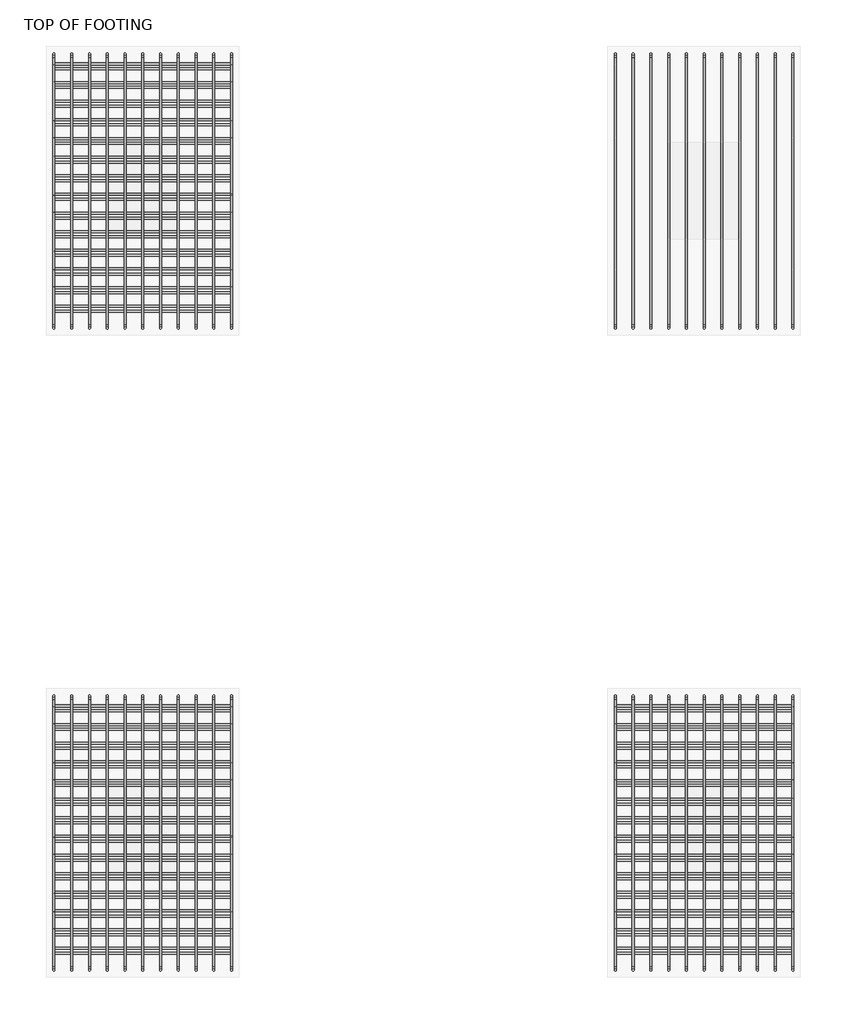
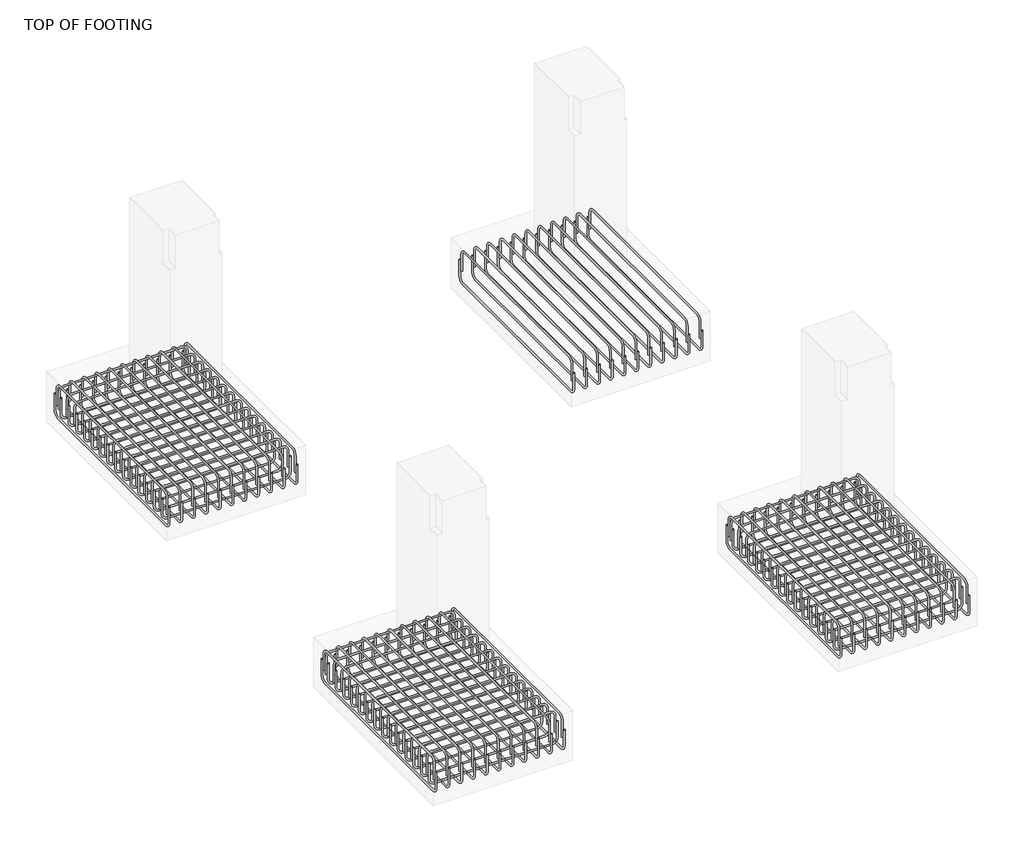
# One storey, part 9 of 11: 14 reinforcing bars.
"""IFC4 building model written with IfcOpenShell, lengths in millimetres."""

from ifc_helpers import new_model, si_unit, point, frame, origin, place, context, project, spatial, polyline, circle_curve, trimmed, segment, composite_curve, source, transform, mapped, element, save
from ifc_brep_helpers import swept_disk

model = new_model("IFC4")

# Units and contexts
model_context = context("Model", 3, world=origin())
ifc_project = project(units=[si_unit("LENGTHUNIT", "METRE", prefix="MILLI")], contexts=[model_context])

# Site, building, storey
site = spatial("IfcSite", under=ifc_project)
building = spatial("IfcBuilding", under=site)
storey = spatial("IfcBuildingStorey", under=building, Name="TOP OF FOOTING", Elevation=-1828.8)

# Reinforcing bars
placement = place(None, origin())
reinforcing_bar_shape = source(origin(), model_context, "Body", "SolidModel", [
    swept_disk(composite_curve([segment(polyline([(5183.7615906, 14549.4712443, -2012.1658531), (5183.7615906, 14549.4712443, -2159.4658531)]), True, "CONTINUOUS"), segment(trimmed(circle_curve(frame((5183.7615906, 14595.8212443, -2159.4658531), z_axis=(1.0, 0.0, 0.0), x_axis=(0.0, -46.349999999998545, 0.0)), 46.35), [point((5183.7615906, 14549.4712443, -2159.4658531))], [point((5183.7615906, 14595.8212443, -2205.8158531))], True, "CARTESIAN"), True, "CONTINUOUS"), segment(polyline([(5183.7615906, 14595.8212443, -2205.8158531), (5183.7615906, 16210.4212443, -2205.8158531)]), True, "CONTINUOUS"), segment(trimmed(circle_curve(frame((5183.7615906, 16210.4212443, -2159.4658531), z_axis=(1.0, 0.0, 0.0), x_axis=(0.0, 0.0, -46.34999999999991)), 46.35), [point((5183.7615906, 16210.4212443, -2205.8158531))], [point((5183.7615906, 16256.7712443, -2159.4658531))], True, "CARTESIAN"), True, "CONTINUOUS"), segment(polyline([(5183.7615906, 16256.7712443, -2159.4658531), (5183.7615906, 16256.7712443, -2012.1658531)]), True, "CONTINUOUS")], self_intersect=False), 6.35),
])
element("IfcReinforcingBar", 1, at=placement, inside=storey, context=model_context, shape_type="MappedRepresentation", body=[
    mapped(reinforcing_bar_shape, transform((0.0, 0.0, 0.0), x_axis=(1.0, 0.0, 0.0), y_axis=(0.0, 1.0, 0.0), z_axis=(0.0, 0.0, 1.0))),
    mapped(reinforcing_bar_shape, transform((-110.73, 0.0, 0.0), x_axis=(1.0, 0.0, 0.0), y_axis=(0.0, 1.0, 0.0), z_axis=(0.0, 0.0, 1.0))),
    mapped(reinforcing_bar_shape, transform((-221.46, 0.0, 0.0), x_axis=(1.0, 0.0, 0.0), y_axis=(0.0, 1.0, 0.0), z_axis=(0.0, 0.0, 1.0))),
    mapped(reinforcing_bar_shape, transform((-332.19, 0.0, 0.0), x_axis=(1.0, 0.0, 0.0), y_axis=(0.0, 1.0, 0.0), z_axis=(0.0, 0.0, 1.0))),
    mapped(reinforcing_bar_shape, transform((-442.92, 0.0, 0.0), x_axis=(1.0, 0.0, 0.0), y_axis=(0.0, 1.0, 0.0), z_axis=(0.0, 0.0, 1.0))),
    mapped(reinforcing_bar_shape, transform((-553.65, 0.0, 0.0), x_axis=(1.0, 0.0, 0.0), y_axis=(0.0, 1.0, 0.0), z_axis=(0.0, 0.0, 1.0))),
    mapped(reinforcing_bar_shape, transform((-664.38, 0.0, 0.0), x_axis=(1.0, 0.0, 0.0), y_axis=(0.0, 1.0, 0.0), z_axis=(0.0, 0.0, 1.0))),
    mapped(reinforcing_bar_shape, transform((-775.11, 0.0, 0.0), x_axis=(1.0, 0.0, 0.0), y_axis=(0.0, 1.0, 0.0), z_axis=(0.0, 0.0, 1.0))),
    mapped(reinforcing_bar_shape, transform((-885.84, 0.0, 0.0), x_axis=(1.0, 0.0, 0.0), y_axis=(0.0, 1.0, 0.0), z_axis=(0.0, 0.0, 1.0))),
    mapped(reinforcing_bar_shape, transform((-996.57, 0.0, 0.0), x_axis=(1.0, 0.0, 0.0), y_axis=(0.0, 1.0, 0.0), z_axis=(0.0, 0.0, 1.0))),
    mapped(reinforcing_bar_shape, transform((-1107.3, 0.0, 0.0), x_axis=(1.0, 0.0, 0.0), y_axis=(0.0, 1.0, 0.0), z_axis=(0.0, 0.0, 1.0))),
])
reinforcing_bar_2_shape = source(origin(), model_context, "Body", "SolidModel", [
    swept_disk(composite_curve([segment(polyline([(4076.4615906, 14577.6603603, -2096.8914539), (4076.4615906, 14577.6603603, -1949.5914539)]), True, "CONTINUOUS"), segment(trimmed(circle_curve(frame((4076.4615906, 14624.0103603, -1949.5914539), z_axis=(-1.0, 0.0, 0.0), x_axis=(0.0, -46.350000000000364, 0.0)), 46.35), [point((4076.4615906, 14577.6603603, -1949.5914539))], [point((4076.4615906, 14624.0103603, -1903.2414539))], True, "CARTESIAN"), True, "CONTINUOUS"), segment(polyline([(4076.4615906, 14624.0103603, -1903.2414539), (4076.4615906, 16181.3238837, -1903.2414539)]), True, "CONTINUOUS"), segment(trimmed(circle_curve(frame((4076.4615906, 16181.3238837, -1949.5914539), z_axis=(-1.0, 0.0, 0.0), x_axis=(0.0, 0.0, 46.350000000000136)), 46.35), [point((4076.4615906, 16181.3238837, -1903.2414539))], [point((4076.4615906, 16227.6738837, -1949.5914539))], True, "CARTESIAN"), True, "CONTINUOUS"), segment(polyline([(4076.4615906, 16227.6738837, -1949.5914539), (4076.4615906, 16227.6738837, -2096.8914539)]), True, "CONTINUOUS")], self_intersect=False), 6.35),
])
element("IfcReinforcingBar", 2, at=placement, inside=storey, context=model_context, shape_type="MappedRepresentation", body=[
    mapped(reinforcing_bar_2_shape, transform((0.0, 0.0, 0.0), x_axis=(1.0, 0.0, 0.0), y_axis=(0.0, 1.0, 0.0), z_axis=(0.0, 0.0, 1.0))),
    mapped(reinforcing_bar_2_shape, transform((110.73, 0.0, 0.0), x_axis=(1.0, 0.0, 0.0), y_axis=(0.0, 1.0, 0.0), z_axis=(0.0, 0.0, 1.0))),
    mapped(reinforcing_bar_2_shape, transform((221.46, 0.0, 0.0), x_axis=(1.0, 0.0, 0.0), y_axis=(0.0, 1.0, 0.0), z_axis=(0.0, 0.0, 1.0))),
    mapped(reinforcing_bar_2_shape, transform((332.19, 0.0, 0.0), x_axis=(1.0, 0.0, 0.0), y_axis=(0.0, 1.0, 0.0), z_axis=(0.0, 0.0, 1.0))),
    mapped(reinforcing_bar_2_shape, transform((442.92, 0.0, 0.0), x_axis=(1.0, 0.0, 0.0), y_axis=(0.0, 1.0, 0.0), z_axis=(0.0, 0.0, 1.0))),
    mapped(reinforcing_bar_2_shape, transform((553.65, 0.0, 0.0), x_axis=(1.0, 0.0, 0.0), y_axis=(0.0, 1.0, 0.0), z_axis=(0.0, 0.0, 1.0))),
    mapped(reinforcing_bar_2_shape, transform((664.38, 0.0, 0.0), x_axis=(1.0, 0.0, 0.0), y_axis=(0.0, 1.0, 0.0), z_axis=(0.0, 0.0, 1.0))),
    mapped(reinforcing_bar_2_shape, transform((775.11, 0.0, 0.0), x_axis=(1.0, 0.0, 0.0), y_axis=(0.0, 1.0, 0.0), z_axis=(0.0, 0.0, 1.0))),
    mapped(reinforcing_bar_2_shape, transform((885.84, 0.0, 0.0), x_axis=(1.0, 0.0, 0.0), y_axis=(0.0, 1.0, 0.0), z_axis=(0.0, 0.0, 1.0))),
    mapped(reinforcing_bar_2_shape, transform((996.57, 0.0, 0.0), x_axis=(1.0, 0.0, 0.0), y_axis=(0.0, 1.0, 0.0), z_axis=(0.0, 0.0, 1.0))),
    mapped(reinforcing_bar_2_shape, transform((1107.3, 0.0, 0.0), x_axis=(1.0, 0.0, 0.0), y_axis=(0.0, 1.0, 0.0), z_axis=(0.0, 0.0, 1.0))),
])
reinforcing_bar_3_shape = source(origin(), model_context, "Body", "SolidModel", [
    swept_disk(composite_curve([segment(polyline([(5183.7615906, 10549.4712443, -2012.1658531), (5183.7615906, 10549.4712443, -2159.4658531)]), True, "CONTINUOUS"), segment(trimmed(circle_curve(frame((5183.7615906, 10595.8212443, -2159.4658531), z_axis=(1.0, 0.0, 0.0), x_axis=(0.0, -46.349999999998545, 0.0)), 46.35), [point((5183.7615906, 10549.4712443, -2159.4658531))], [point((5183.7615906, 10595.8212443, -2205.8158531))], True, "CARTESIAN"), True, "CONTINUOUS"), segment(polyline([(5183.7615906, 10595.8212443, -2205.8158531), (5183.7615906, 12210.4212443, -2205.8158531)]), True, "CONTINUOUS"), segment(trimmed(circle_curve(frame((5183.7615906, 12210.4212443, -2159.4658531), z_axis=(1.0, 0.0, 0.0), x_axis=(0.0, 0.0, -46.34999999999991)), 46.35), [point((5183.7615906, 12210.4212443, -2205.8158531))], [point((5183.7615906, 12256.7712443, -2159.4658531))], True, "CARTESIAN"), True, "CONTINUOUS"), segment(polyline([(5183.7615906, 12256.7712443, -2159.4658531), (5183.7615906, 12256.7712443, -2012.1658531)]), True, "CONTINUOUS")], self_intersect=False), 6.35),
])
element("IfcReinforcingBar", 3, at=placement, inside=storey, context=model_context, shape_type="MappedRepresentation", body=[
    mapped(reinforcing_bar_3_shape, transform((0.0, 0.0, 0.0), x_axis=(1.0, 0.0, 0.0), y_axis=(0.0, 1.0, 0.0), z_axis=(0.0, 0.0, 1.0))),
    mapped(reinforcing_bar_3_shape, transform((-110.73, 0.0, 0.0), x_axis=(1.0, 0.0, 0.0), y_axis=(0.0, 1.0, 0.0), z_axis=(0.0, 0.0, 1.0))),
    mapped(reinforcing_bar_3_shape, transform((-221.46, 0.0, 0.0), x_axis=(1.0, 0.0, 0.0), y_axis=(0.0, 1.0, 0.0), z_axis=(0.0, 0.0, 1.0))),
    mapped(reinforcing_bar_3_shape, transform((-332.19, 0.0, 0.0), x_axis=(1.0, 0.0, 0.0), y_axis=(0.0, 1.0, 0.0), z_axis=(0.0, 0.0, 1.0))),
    mapped(reinforcing_bar_3_shape, transform((-442.92, 0.0, 0.0), x_axis=(1.0, 0.0, 0.0), y_axis=(0.0, 1.0, 0.0), z_axis=(0.0, 0.0, 1.0))),
    mapped(reinforcing_bar_3_shape, transform((-553.65, 0.0, 0.0), x_axis=(1.0, 0.0, 0.0), y_axis=(0.0, 1.0, 0.0), z_axis=(0.0, 0.0, 1.0))),
    mapped(reinforcing_bar_3_shape, transform((-664.38, 0.0, 0.0), x_axis=(1.0, 0.0, 0.0), y_axis=(0.0, 1.0, 0.0), z_axis=(0.0, 0.0, 1.0))),
    mapped(reinforcing_bar_3_shape, transform((-775.11, 0.0, 0.0), x_axis=(1.0, 0.0, 0.0), y_axis=(0.0, 1.0, 0.0), z_axis=(0.0, 0.0, 1.0))),
    mapped(reinforcing_bar_3_shape, transform((-885.84, 0.0, 0.0), x_axis=(1.0, 0.0, 0.0), y_axis=(0.0, 1.0, 0.0), z_axis=(0.0, 0.0, 1.0))),
    mapped(reinforcing_bar_3_shape, transform((-996.57, 0.0, 0.0), x_axis=(1.0, 0.0, 0.0), y_axis=(0.0, 1.0, 0.0), z_axis=(0.0, 0.0, 1.0))),
    mapped(reinforcing_bar_3_shape, transform((-1107.3, 0.0, 0.0), x_axis=(1.0, 0.0, 0.0), y_axis=(0.0, 1.0, 0.0), z_axis=(0.0, 0.0, 1.0))),
])
reinforcing_bar_4_shape = source(origin(), model_context, "Body", "SolidModel", [
    swept_disk(composite_curve([segment(polyline([(4076.4615906, 10577.6603603, -2096.8914539), (4076.4615906, 10577.6603603, -1949.5914539)]), True, "CONTINUOUS"), segment(trimmed(circle_curve(frame((4076.4615906, 10624.0103603, -1949.5914539), z_axis=(-1.0, 0.0, 0.0), x_axis=(0.0, -46.350000000000364, 0.0)), 46.35), [point((4076.4615906, 10577.6603603, -1949.5914539))], [point((4076.4615906, 10624.0103603, -1903.2414539))], True, "CARTESIAN"), True, "CONTINUOUS"), segment(polyline([(4076.4615906, 10624.0103603, -1903.2414539), (4076.4615906, 12181.3238837, -1903.2414539)]), True, "CONTINUOUS"), segment(trimmed(circle_curve(frame((4076.4615906, 12181.3238837, -1949.5914539), z_axis=(-1.0, 0.0, 0.0), x_axis=(0.0, 0.0, 46.350000000000136)), 46.35), [point((4076.4615906, 12181.3238837, -1903.2414539))], [point((4076.4615906, 12227.6738837, -1949.5914539))], True, "CARTESIAN"), True, "CONTINUOUS"), segment(polyline([(4076.4615906, 12227.6738837, -1949.5914539), (4076.4615906, 12227.6738837, -2096.8914539)]), True, "CONTINUOUS")], self_intersect=False), 6.35),
])
element("IfcReinforcingBar", 4, at=placement, inside=storey, context=model_context, shape_type="MappedRepresentation", body=[
    mapped(reinforcing_bar_4_shape, transform((0.0, 0.0, 0.0), x_axis=(1.0, 0.0, 0.0), y_axis=(0.0, 1.0, 0.0), z_axis=(0.0, 0.0, 1.0))),
    mapped(reinforcing_bar_4_shape, transform((110.73, 0.0, 0.0), x_axis=(1.0, 0.0, 0.0), y_axis=(0.0, 1.0, 0.0), z_axis=(0.0, 0.0, 1.0))),
    mapped(reinforcing_bar_4_shape, transform((221.46, 0.0, 0.0), x_axis=(1.0, 0.0, 0.0), y_axis=(0.0, 1.0, 0.0), z_axis=(0.0, 0.0, 1.0))),
    mapped(reinforcing_bar_4_shape, transform((332.19, 0.0, 0.0), x_axis=(1.0, 0.0, 0.0), y_axis=(0.0, 1.0, 0.0), z_axis=(0.0, 0.0, 1.0))),
    mapped(reinforcing_bar_4_shape, transform((442.92, 0.0, 0.0), x_axis=(1.0, 0.0, 0.0), y_axis=(0.0, 1.0, 0.0), z_axis=(0.0, 0.0, 1.0))),
    mapped(reinforcing_bar_4_shape, transform((553.65, 0.0, 0.0), x_axis=(1.0, 0.0, 0.0), y_axis=(0.0, 1.0, 0.0), z_axis=(0.0, 0.0, 1.0))),
    mapped(reinforcing_bar_4_shape, transform((664.38, 0.0, 0.0), x_axis=(1.0, 0.0, 0.0), y_axis=(0.0, 1.0, 0.0), z_axis=(0.0, 0.0, 1.0))),
    mapped(reinforcing_bar_4_shape, transform((775.11, 0.0, 0.0), x_axis=(1.0, 0.0, 0.0), y_axis=(0.0, 1.0, 0.0), z_axis=(0.0, 0.0, 1.0))),
    mapped(reinforcing_bar_4_shape, transform((885.84, 0.0, 0.0), x_axis=(1.0, 0.0, 0.0), y_axis=(0.0, 1.0, 0.0), z_axis=(0.0, 0.0, 1.0))),
    mapped(reinforcing_bar_4_shape, transform((996.57, 0.0, 0.0), x_axis=(1.0, 0.0, 0.0), y_axis=(0.0, 1.0, 0.0), z_axis=(0.0, 0.0, 1.0))),
    mapped(reinforcing_bar_4_shape, transform((1107.3, 0.0, 0.0), x_axis=(1.0, 0.0, 0.0), y_axis=(0.0, 1.0, 0.0), z_axis=(0.0, 0.0, 1.0))),
])
reinforcing_bar_5_shape = source(origin(), model_context, "Body", "SolidModel", [
    swept_disk(composite_curve([segment(polyline([(4076.4615906, 10653.1930221, -1996.7664426), (4076.4615906, 10653.1930221, -2144.0664426)]), True, "CONTINUOUS"), segment(trimmed(circle_curve(frame((4122.8115906, 10653.1930221, -2144.0664426), z_axis=(0.0, -1.0, 0.0), x_axis=(-46.350000000000364, 0.0, 0.0)), 46.35), [point((4076.4615906, 10653.1930221, -2144.0664426))], [point((4122.8115906, 10653.1930221, -2190.4164426))], True, "CARTESIAN"), True, "CONTINUOUS"), segment(polyline([(4122.8115906, 10653.1930221, -2190.4164426), (5137.4115906, 10653.1930221, -2190.4164426)]), True, "CONTINUOUS"), segment(trimmed(circle_curve(frame((5137.4115906, 10653.1930221, -2144.0664426), z_axis=(0.0, -1.0, 0.0), x_axis=(0.0, 0.0, -46.350000000000364)), 46.35), [point((5137.4115906, 10653.1930221, -2190.4164426))], [point((5183.7615906, 10653.1930221, -2144.0664426))], True, "CARTESIAN"), True, "CONTINUOUS"), segment(polyline([(5183.7615906, 10653.1930221, -2144.0664426), (5183.7615906, 10653.1930221, -1996.7664426)]), True, "CONTINUOUS")], self_intersect=False), 6.35),
])
element("IfcReinforcingBar", 5, at=placement, inside=storey, context=model_context, shape_type="MappedRepresentation", body=[
    mapped(reinforcing_bar_5_shape, transform((0.0, 0.0, 0.0), x_axis=(1.0, 0.0, 0.0), y_axis=(0.0, 1.0, 0.0), z_axis=(0.0, 0.0, 1.0))),
    mapped(reinforcing_bar_5_shape, transform((0.0, 116.2744005, 0.0), x_axis=(1.0, 0.0, 0.0), y_axis=(0.0, 1.0, 0.0), z_axis=(0.0, 0.0, 1.0))),
    mapped(reinforcing_bar_5_shape, transform((0.0, 232.5488009, 0.0), x_axis=(1.0, 0.0, 0.0), y_axis=(0.0, 1.0, 0.0), z_axis=(0.0, 0.0, 1.0))),
    mapped(reinforcing_bar_5_shape, transform((0.0, 348.8232014, 0.0), x_axis=(1.0, 0.0, 0.0), y_axis=(0.0, 1.0, 0.0), z_axis=(0.0, 0.0, 1.0))),
    mapped(reinforcing_bar_5_shape, transform((0.0, 465.0976018, 0.0), x_axis=(1.0, 0.0, 0.0), y_axis=(0.0, 1.0, 0.0), z_axis=(0.0, 0.0, 1.0))),
    mapped(reinforcing_bar_5_shape, transform((0.0, 581.3720023, 0.0), x_axis=(1.0, 0.0, 0.0), y_axis=(0.0, 1.0, 0.0), z_axis=(0.0, 0.0, 1.0))),
    mapped(reinforcing_bar_5_shape, transform((0.0, 697.6464027, 0.0), x_axis=(1.0, 0.0, 0.0), y_axis=(0.0, 1.0, 0.0), z_axis=(0.0, 0.0, 1.0))),
    mapped(reinforcing_bar_5_shape, transform((0.0, 813.9208032, 0.0), x_axis=(1.0, 0.0, 0.0), y_axis=(0.0, 1.0, 0.0), z_axis=(0.0, 0.0, 1.0))),
    mapped(reinforcing_bar_5_shape, transform((0.0, 930.1952036, 0.0), x_axis=(1.0, 0.0, 0.0), y_axis=(0.0, 1.0, 0.0), z_axis=(0.0, 0.0, 1.0))),
    mapped(reinforcing_bar_5_shape, transform((0.0, 1046.4696041, 0.0), x_axis=(1.0, 0.0, 0.0), y_axis=(0.0, 1.0, 0.0), z_axis=(0.0, 0.0, 1.0))),
    mapped(reinforcing_bar_5_shape, transform((0.0, 1162.7440045, 0.0), x_axis=(1.0, 0.0, 0.0), y_axis=(0.0, 1.0, 0.0), z_axis=(0.0, 0.0, 1.0))),
    mapped(reinforcing_bar_5_shape, transform((0.0, 1279.018405, 0.0), x_axis=(1.0, 0.0, 0.0), y_axis=(0.0, 1.0, 0.0), z_axis=(0.0, 0.0, 1.0))),
    mapped(reinforcing_bar_5_shape, transform((0.0, 1395.2928054, 0.0), x_axis=(1.0, 0.0, 0.0), y_axis=(0.0, 1.0, 0.0), z_axis=(0.0, 0.0, 1.0))),
    mapped(reinforcing_bar_5_shape, transform((0.0, 1511.5672059, 0.0), x_axis=(1.0, 0.0, 0.0), y_axis=(0.0, 1.0, 0.0), z_axis=(0.0, 0.0, 1.0))),
])
reinforcing_bar_6_shape = source(origin(), model_context, "Body", "SolidModel", [
    swept_disk(composite_curve([segment(polyline([(4076.4615906, 12194.4257435, -2114.1958609), (4076.4615906, 12194.4257435, -1966.8958609)]), True, "CONTINUOUS"), segment(trimmed(circle_curve(frame((4122.8115906, 12194.4257435, -1966.8958609), z_axis=(0.0, 1.0, 0.0), x_axis=(-46.350000000000364, 0.0, 0.0)), 46.35), [point((4076.4615906, 12194.4257435, -1966.8958609))], [point((4122.8115906, 12194.4257435, -1920.5458609))], True, "CARTESIAN"), True, "CONTINUOUS"), segment(polyline([(4122.8115906, 12194.4257435, -1920.5458609), (5137.4115906, 12194.4257435, -1920.5458609)]), True, "CONTINUOUS"), segment(trimmed(circle_curve(frame((5137.4115906, 12194.4257435, -1966.8958609), z_axis=(0.0, 1.0, 0.0), x_axis=(0.0, 0.0, 46.34999999999991)), 46.35), [point((5137.4115906, 12194.4257435, -1920.5458609))], [point((5183.7615906, 12194.4257435, -1966.8958609))], True, "CARTESIAN"), True, "CONTINUOUS"), segment(polyline([(5183.7615906, 12194.4257435, -1966.8958609), (5183.7615906, 12194.4257435, -2114.1958609)]), True, "CONTINUOUS")], self_intersect=False), 6.35),
])
element("IfcReinforcingBar", 6, at=placement, inside=storey, context=model_context, shape_type="MappedRepresentation", body=[
    mapped(reinforcing_bar_6_shape, transform((0.0, 0.0, 0.0), x_axis=(1.0, 0.0, 0.0), y_axis=(0.0, 1.0, 0.0), z_axis=(0.0, 0.0, 1.0))),
    mapped(reinforcing_bar_6_shape, transform((0.0, -116.1057918, 0.0), x_axis=(1.0, 0.0, 0.0), y_axis=(0.0, 1.0, 0.0), z_axis=(0.0, 0.0, 1.0))),
    mapped(reinforcing_bar_6_shape, transform((0.0, -232.2115836, 0.0), x_axis=(1.0, 0.0, 0.0), y_axis=(0.0, 1.0, 0.0), z_axis=(0.0, 0.0, 1.0))),
    mapped(reinforcing_bar_6_shape, transform((0.0, -348.3173754, 0.0), x_axis=(1.0, 0.0, 0.0), y_axis=(0.0, 1.0, 0.0), z_axis=(0.0, 0.0, 1.0))),
    mapped(reinforcing_bar_6_shape, transform((0.0, -464.4231672, 0.0), x_axis=(1.0, 0.0, 0.0), y_axis=(0.0, 1.0, 0.0), z_axis=(0.0, 0.0, 1.0))),
    mapped(reinforcing_bar_6_shape, transform((0.0, -580.528959, 0.0), x_axis=(1.0, 0.0, 0.0), y_axis=(0.0, 1.0, 0.0), z_axis=(0.0, 0.0, 1.0))),
    mapped(reinforcing_bar_6_shape, transform((0.0, -696.6347508, 0.0), x_axis=(1.0, 0.0, 0.0), y_axis=(0.0, 1.0, 0.0), z_axis=(0.0, 0.0, 1.0))),
    mapped(reinforcing_bar_6_shape, transform((0.0, -812.7405426, 0.0), x_axis=(1.0, 0.0, 0.0), y_axis=(0.0, 1.0, 0.0), z_axis=(0.0, 0.0, 1.0))),
    mapped(reinforcing_bar_6_shape, transform((0.0, -928.8463344, 0.0), x_axis=(1.0, 0.0, 0.0), y_axis=(0.0, 1.0, 0.0), z_axis=(0.0, 0.0, 1.0))),
    mapped(reinforcing_bar_6_shape, transform((0.0, -1044.9521262, 0.0), x_axis=(1.0, 0.0, 0.0), y_axis=(0.0, 1.0, 0.0), z_axis=(0.0, 0.0, 1.0))),
    mapped(reinforcing_bar_6_shape, transform((0.0, -1161.057918, 0.0), x_axis=(1.0, 0.0, 0.0), y_axis=(0.0, 1.0, 0.0), z_axis=(0.0, 0.0, 1.0))),
    mapped(reinforcing_bar_6_shape, transform((0.0, -1277.1637098, 0.0), x_axis=(1.0, 0.0, 0.0), y_axis=(0.0, 1.0, 0.0), z_axis=(0.0, 0.0, 1.0))),
    mapped(reinforcing_bar_6_shape, transform((0.0, -1393.2695016, 0.0), x_axis=(1.0, 0.0, 0.0), y_axis=(0.0, 1.0, 0.0), z_axis=(0.0, 0.0, 1.0))),
    mapped(reinforcing_bar_6_shape, transform((0.0, -1509.3752934, 0.0), x_axis=(1.0, 0.0, 0.0), y_axis=(0.0, 1.0, 0.0), z_axis=(0.0, 0.0, 1.0))),
])
reinforcing_bar_7_shape = source(origin(), model_context, "Body", "SolidModel", [
    swept_disk(composite_curve([segment(polyline([(1683.7615906, 14549.4712443, -2012.1658531), (1683.7615906, 14549.4712443, -2159.4658531)]), True, "CONTINUOUS"), segment(trimmed(circle_curve(frame((1683.7615906, 14595.8212443, -2159.4658531), z_axis=(1.0, 0.0, 0.0), x_axis=(0.0, -46.349999999998545, 0.0)), 46.35), [point((1683.7615906, 14549.4712443, -2159.4658531))], [point((1683.7615906, 14595.8212443, -2205.8158531))], True, "CARTESIAN"), True, "CONTINUOUS"), segment(polyline([(1683.7615906, 14595.8212443, -2205.8158531), (1683.7615906, 16210.4212443, -2205.8158531)]), True, "CONTINUOUS"), segment(trimmed(circle_curve(frame((1683.7615906, 16210.4212443, -2159.4658531), z_axis=(1.0, 0.0, 0.0), x_axis=(0.0, 0.0, -46.34999999999991)), 46.35), [point((1683.7615906, 16210.4212443, -2205.8158531))], [point((1683.7615906, 16256.7712443, -2159.4658531))], True, "CARTESIAN"), True, "CONTINUOUS"), segment(polyline([(1683.7615906, 16256.7712443, -2159.4658531), (1683.7615906, 16256.7712443, -2012.1658531)]), True, "CONTINUOUS")], self_intersect=False), 6.35),
])
element("IfcReinforcingBar", 7, at=placement, inside=storey, context=model_context, shape_type="MappedRepresentation", body=[
    mapped(reinforcing_bar_7_shape, transform((0.0, 0.0, 0.0), x_axis=(1.0, 0.0, 0.0), y_axis=(0.0, 1.0, 0.0), z_axis=(0.0, 0.0, 1.0))),
    mapped(reinforcing_bar_7_shape, transform((-110.73, 0.0, 0.0), x_axis=(1.0, 0.0, 0.0), y_axis=(0.0, 1.0, 0.0), z_axis=(0.0, 0.0, 1.0))),
    mapped(reinforcing_bar_7_shape, transform((-221.46, 0.0, 0.0), x_axis=(1.0, 0.0, 0.0), y_axis=(0.0, 1.0, 0.0), z_axis=(0.0, 0.0, 1.0))),
    mapped(reinforcing_bar_7_shape, transform((-332.19, 0.0, 0.0), x_axis=(1.0, 0.0, 0.0), y_axis=(0.0, 1.0, 0.0), z_axis=(0.0, 0.0, 1.0))),
    mapped(reinforcing_bar_7_shape, transform((-442.92, 0.0, 0.0), x_axis=(1.0, 0.0, 0.0), y_axis=(0.0, 1.0, 0.0), z_axis=(0.0, 0.0, 1.0))),
    mapped(reinforcing_bar_7_shape, transform((-553.65, 0.0, 0.0), x_axis=(1.0, 0.0, 0.0), y_axis=(0.0, 1.0, 0.0), z_axis=(0.0, 0.0, 1.0))),
    mapped(reinforcing_bar_7_shape, transform((-664.38, 0.0, 0.0), x_axis=(1.0, 0.0, 0.0), y_axis=(0.0, 1.0, 0.0), z_axis=(0.0, 0.0, 1.0))),
    mapped(reinforcing_bar_7_shape, transform((-775.11, 0.0, 0.0), x_axis=(1.0, 0.0, 0.0), y_axis=(0.0, 1.0, 0.0), z_axis=(0.0, 0.0, 1.0))),
    mapped(reinforcing_bar_7_shape, transform((-885.84, 0.0, 0.0), x_axis=(1.0, 0.0, 0.0), y_axis=(0.0, 1.0, 0.0), z_axis=(0.0, 0.0, 1.0))),
    mapped(reinforcing_bar_7_shape, transform((-996.57, 0.0, 0.0), x_axis=(1.0, 0.0, 0.0), y_axis=(0.0, 1.0, 0.0), z_axis=(0.0, 0.0, 1.0))),
    mapped(reinforcing_bar_7_shape, transform((-1107.3, 0.0, 0.0), x_axis=(1.0, 0.0, 0.0), y_axis=(0.0, 1.0, 0.0), z_axis=(0.0, 0.0, 1.0))),
])
reinforcing_bar_8_shape = source(origin(), model_context, "Body", "SolidModel", [
    swept_disk(composite_curve([segment(polyline([(576.4615906, 14577.6603603, -2096.8914539), (576.4615906, 14577.6603603, -1949.5914539)]), True, "CONTINUOUS"), segment(trimmed(circle_curve(frame((576.4615906, 14624.0103603, -1949.5914539), z_axis=(-1.0, 0.0, 0.0), x_axis=(0.0, -46.350000000000364, 0.0)), 46.35), [point((576.4615906, 14577.6603603, -1949.5914539))], [point((576.4615906, 14624.0103603, -1903.2414539))], True, "CARTESIAN"), True, "CONTINUOUS"), segment(polyline([(576.4615906, 14624.0103603, -1903.2414539), (576.4615906, 16181.3238837, -1903.2414539)]), True, "CONTINUOUS"), segment(trimmed(circle_curve(frame((576.4615906, 16181.3238837, -1949.5914539), z_axis=(-1.0, 0.0, 0.0), x_axis=(0.0, 0.0, 46.350000000000136)), 46.35), [point((576.4615906, 16181.3238837, -1903.2414539))], [point((576.4615906, 16227.6738837, -1949.5914539))], True, "CARTESIAN"), True, "CONTINUOUS"), segment(polyline([(576.4615906, 16227.6738837, -1949.5914539), (576.4615906, 16227.6738837, -2096.8914539)]), True, "CONTINUOUS")], self_intersect=False), 6.35),
])
element("IfcReinforcingBar", 8, at=placement, inside=storey, context=model_context, shape_type="MappedRepresentation", body=[
    mapped(reinforcing_bar_8_shape, transform((0.0, 0.0, 0.0), x_axis=(1.0, 0.0, 0.0), y_axis=(0.0, 1.0, 0.0), z_axis=(0.0, 0.0, 1.0))),
    mapped(reinforcing_bar_8_shape, transform((110.73, 0.0, 0.0), x_axis=(1.0, 0.0, 0.0), y_axis=(0.0, 1.0, 0.0), z_axis=(0.0, 0.0, 1.0))),
    mapped(reinforcing_bar_8_shape, transform((221.46, 0.0, 0.0), x_axis=(1.0, 0.0, 0.0), y_axis=(0.0, 1.0, 0.0), z_axis=(0.0, 0.0, 1.0))),
    mapped(reinforcing_bar_8_shape, transform((332.19, 0.0, 0.0), x_axis=(1.0, 0.0, 0.0), y_axis=(0.0, 1.0, 0.0), z_axis=(0.0, 0.0, 1.0))),
    mapped(reinforcing_bar_8_shape, transform((442.92, 0.0, 0.0), x_axis=(1.0, 0.0, 0.0), y_axis=(0.0, 1.0, 0.0), z_axis=(0.0, 0.0, 1.0))),
    mapped(reinforcing_bar_8_shape, transform((553.65, 0.0, 0.0), x_axis=(1.0, 0.0, 0.0), y_axis=(0.0, 1.0, 0.0), z_axis=(0.0, 0.0, 1.0))),
    mapped(reinforcing_bar_8_shape, transform((664.38, 0.0, 0.0), x_axis=(1.0, 0.0, 0.0), y_axis=(0.0, 1.0, 0.0), z_axis=(0.0, 0.0, 1.0))),
    mapped(reinforcing_bar_8_shape, transform((775.11, 0.0, 0.0), x_axis=(1.0, 0.0, 0.0), y_axis=(0.0, 1.0, 0.0), z_axis=(0.0, 0.0, 1.0))),
    mapped(reinforcing_bar_8_shape, transform((885.84, 0.0, 0.0), x_axis=(1.0, 0.0, 0.0), y_axis=(0.0, 1.0, 0.0), z_axis=(0.0, 0.0, 1.0))),
    mapped(reinforcing_bar_8_shape, transform((996.57, 0.0, 0.0), x_axis=(1.0, 0.0, 0.0), y_axis=(0.0, 1.0, 0.0), z_axis=(0.0, 0.0, 1.0))),
    mapped(reinforcing_bar_8_shape, transform((1107.3, 0.0, 0.0), x_axis=(1.0, 0.0, 0.0), y_axis=(0.0, 1.0, 0.0), z_axis=(0.0, 0.0, 1.0))),
])
reinforcing_bar_9_shape = source(origin(), model_context, "Body", "SolidModel", [
    swept_disk(composite_curve([segment(polyline([(576.4615906, 14653.1930221, -1996.7664426), (576.4615906, 14653.1930221, -2144.0664426)]), True, "CONTINUOUS"), segment(trimmed(circle_curve(frame((622.8115906, 14653.1930221, -2144.0664426), z_axis=(0.0, -1.0, 0.0), x_axis=(-46.35000000000002, 0.0, 0.0)), 46.35), [point((576.4615906, 14653.1930221, -2144.0664426))], [point((622.8115906, 14653.1930221, -2190.4164426))], True, "CARTESIAN"), True, "CONTINUOUS"), segment(polyline([(622.8115906, 14653.1930221, -2190.4164426), (1637.4115906, 14653.1930221, -2190.4164426)]), True, "CONTINUOUS"), segment(trimmed(circle_curve(frame((1637.4115906, 14653.1930221, -2144.0664426), z_axis=(0.0, -1.0, 0.0), x_axis=(0.0, 0.0, -46.350000000000364)), 46.35), [point((1637.4115906, 14653.1930221, -2190.4164426))], [point((1683.7615906, 14653.1930221, -2144.0664426))], True, "CARTESIAN"), True, "CONTINUOUS"), segment(polyline([(1683.7615906, 14653.1930221, -2144.0664426), (1683.7615906, 14653.1930221, -1996.7664426)]), True, "CONTINUOUS")], self_intersect=False), 6.35),
])
element("IfcReinforcingBar", 9, at=placement, inside=storey, context=model_context, shape_type="MappedRepresentation", body=[
    mapped(reinforcing_bar_9_shape, transform((0.0, 0.0, 0.0), x_axis=(1.0, 0.0, 0.0), y_axis=(0.0, 1.0, 0.0), z_axis=(0.0, 0.0, 1.0))),
    mapped(reinforcing_bar_9_shape, transform((0.0, 116.2744005, 0.0), x_axis=(1.0, 0.0, 0.0), y_axis=(0.0, 1.0, 0.0), z_axis=(0.0, 0.0, 1.0))),
    mapped(reinforcing_bar_9_shape, transform((0.0, 232.5488009, 0.0), x_axis=(1.0, 0.0, 0.0), y_axis=(0.0, 1.0, 0.0), z_axis=(0.0, 0.0, 1.0))),
    mapped(reinforcing_bar_9_shape, transform((0.0, 348.8232014, 0.0), x_axis=(1.0, 0.0, 0.0), y_axis=(0.0, 1.0, 0.0), z_axis=(0.0, 0.0, 1.0))),
    mapped(reinforcing_bar_9_shape, transform((0.0, 465.0976018, 0.0), x_axis=(1.0, 0.0, 0.0), y_axis=(0.0, 1.0, 0.0), z_axis=(0.0, 0.0, 1.0))),
    mapped(reinforcing_bar_9_shape, transform((0.0, 581.3720023, 0.0), x_axis=(1.0, 0.0, 0.0), y_axis=(0.0, 1.0, 0.0), z_axis=(0.0, 0.0, 1.0))),
    mapped(reinforcing_bar_9_shape, transform((0.0, 697.6464027, 0.0), x_axis=(1.0, 0.0, 0.0), y_axis=(0.0, 1.0, 0.0), z_axis=(0.0, 0.0, 1.0))),
    mapped(reinforcing_bar_9_shape, transform((0.0, 813.9208032, 0.0), x_axis=(1.0, 0.0, 0.0), y_axis=(0.0, 1.0, 0.0), z_axis=(0.0, 0.0, 1.0))),
    mapped(reinforcing_bar_9_shape, transform((0.0, 930.1952036, 0.0), x_axis=(1.0, 0.0, 0.0), y_axis=(0.0, 1.0, 0.0), z_axis=(0.0, 0.0, 1.0))),
    mapped(reinforcing_bar_9_shape, transform((0.0, 1046.4696041, 0.0), x_axis=(1.0, 0.0, 0.0), y_axis=(0.0, 1.0, 0.0), z_axis=(0.0, 0.0, 1.0))),
    mapped(reinforcing_bar_9_shape, transform((0.0, 1162.7440045, 0.0), x_axis=(1.0, 0.0, 0.0), y_axis=(0.0, 1.0, 0.0), z_axis=(0.0, 0.0, 1.0))),
    mapped(reinforcing_bar_9_shape, transform((0.0, 1279.018405, 0.0), x_axis=(1.0, 0.0, 0.0), y_axis=(0.0, 1.0, 0.0), z_axis=(0.0, 0.0, 1.0))),
    mapped(reinforcing_bar_9_shape, transform((0.0, 1395.2928054, 0.0), x_axis=(1.0, 0.0, 0.0), y_axis=(0.0, 1.0, 0.0), z_axis=(0.0, 0.0, 1.0))),
    mapped(reinforcing_bar_9_shape, transform((0.0, 1511.5672059, 0.0), x_axis=(1.0, 0.0, 0.0), y_axis=(0.0, 1.0, 0.0), z_axis=(0.0, 0.0, 1.0))),
])
reinforcing_bar_10_shape = source(origin(), model_context, "Body", "SolidModel", [
    swept_disk(composite_curve([segment(polyline([(576.4615906, 16194.4257435, -2114.1958609), (576.4615906, 16194.4257435, -1966.8958609)]), True, "CONTINUOUS"), segment(trimmed(circle_curve(frame((622.8115906, 16194.4257435, -1966.8958609), z_axis=(0.0, 1.0, 0.0), x_axis=(-46.35000000000002, 0.0, 0.0)), 46.35), [point((576.4615906, 16194.4257435, -1966.8958609))], [point((622.8115906, 16194.4257435, -1920.5458609))], True, "CARTESIAN"), True, "CONTINUOUS"), segment(polyline([(622.8115906, 16194.4257435, -1920.5458609), (1637.4115906, 16194.4257435, -1920.5458609)]), True, "CONTINUOUS"), segment(trimmed(circle_curve(frame((1637.4115906, 16194.4257435, -1966.8958609), z_axis=(0.0, 1.0, 0.0), x_axis=(0.0, 0.0, 46.34999999999991)), 46.35), [point((1637.4115906, 16194.4257435, -1920.5458609))], [point((1683.7615906, 16194.4257435, -1966.8958609))], True, "CARTESIAN"), True, "CONTINUOUS"), segment(polyline([(1683.7615906, 16194.4257435, -1966.8958609), (1683.7615906, 16194.4257435, -2114.1958609)]), True, "CONTINUOUS")], self_intersect=False), 6.35),
])
element("IfcReinforcingBar", 10, at=placement, inside=storey, context=model_context, shape_type="MappedRepresentation", body=[
    mapped(reinforcing_bar_10_shape, transform((0.0, 0.0, 0.0), x_axis=(1.0, 0.0, 0.0), y_axis=(0.0, 1.0, 0.0), z_axis=(0.0, 0.0, 1.0))),
    mapped(reinforcing_bar_10_shape, transform((0.0, -116.1057918, 0.0), x_axis=(1.0, 0.0, 0.0), y_axis=(0.0, 1.0, 0.0), z_axis=(0.0, 0.0, 1.0))),
    mapped(reinforcing_bar_10_shape, transform((0.0, -232.2115836, 0.0), x_axis=(1.0, 0.0, 0.0), y_axis=(0.0, 1.0, 0.0), z_axis=(0.0, 0.0, 1.0))),
    mapped(reinforcing_bar_10_shape, transform((0.0, -348.3173754, 0.0), x_axis=(1.0, 0.0, 0.0), y_axis=(0.0, 1.0, 0.0), z_axis=(0.0, 0.0, 1.0))),
    mapped(reinforcing_bar_10_shape, transform((0.0, -464.4231672, 0.0), x_axis=(1.0, 0.0, 0.0), y_axis=(0.0, 1.0, 0.0), z_axis=(0.0, 0.0, 1.0))),
    mapped(reinforcing_bar_10_shape, transform((0.0, -580.528959, 0.0), x_axis=(1.0, 0.0, 0.0), y_axis=(0.0, 1.0, 0.0), z_axis=(0.0, 0.0, 1.0))),
    mapped(reinforcing_bar_10_shape, transform((0.0, -696.6347508, 0.0), x_axis=(1.0, 0.0, 0.0), y_axis=(0.0, 1.0, 0.0), z_axis=(0.0, 0.0, 1.0))),
    mapped(reinforcing_bar_10_shape, transform((0.0, -812.7405426, 0.0), x_axis=(1.0, 0.0, 0.0), y_axis=(0.0, 1.0, 0.0), z_axis=(0.0, 0.0, 1.0))),
    mapped(reinforcing_bar_10_shape, transform((0.0, -928.8463344, 0.0), x_axis=(1.0, 0.0, 0.0), y_axis=(0.0, 1.0, 0.0), z_axis=(0.0, 0.0, 1.0))),
    mapped(reinforcing_bar_10_shape, transform((0.0, -1044.9521262, 0.0), x_axis=(1.0, 0.0, 0.0), y_axis=(0.0, 1.0, 0.0), z_axis=(0.0, 0.0, 1.0))),
    mapped(reinforcing_bar_10_shape, transform((0.0, -1161.057918, 0.0), x_axis=(1.0, 0.0, 0.0), y_axis=(0.0, 1.0, 0.0), z_axis=(0.0, 0.0, 1.0))),
    mapped(reinforcing_bar_10_shape, transform((0.0, -1277.1637098, 0.0), x_axis=(1.0, 0.0, 0.0), y_axis=(0.0, 1.0, 0.0), z_axis=(0.0, 0.0, 1.0))),
    mapped(reinforcing_bar_10_shape, transform((0.0, -1393.2695016, 0.0), x_axis=(1.0, 0.0, 0.0), y_axis=(0.0, 1.0, 0.0), z_axis=(0.0, 0.0, 1.0))),
    mapped(reinforcing_bar_10_shape, transform((0.0, -1509.3752934, 0.0), x_axis=(1.0, 0.0, 0.0), y_axis=(0.0, 1.0, 0.0), z_axis=(0.0, 0.0, 1.0))),
])
reinforcing_bar_11_shape = source(origin(), model_context, "Body", "SolidModel", [
    swept_disk(composite_curve([segment(polyline([(1683.7615906, 10549.4712443, -2012.1658531), (1683.7615906, 10549.4712443, -2159.4658531)]), True, "CONTINUOUS"), segment(trimmed(circle_curve(frame((1683.7615906, 10595.8212443, -2159.4658531), z_axis=(1.0, 0.0, 0.0), x_axis=(0.0, -46.349999999998545, 0.0)), 46.35), [point((1683.7615906, 10549.4712443, -2159.4658531))], [point((1683.7615906, 10595.8212443, -2205.8158531))], True, "CARTESIAN"), True, "CONTINUOUS"), segment(polyline([(1683.7615906, 10595.8212443, -2205.8158531), (1683.7615906, 12210.4212443, -2205.8158531)]), True, "CONTINUOUS"), segment(trimmed(circle_curve(frame((1683.7615906, 12210.4212443, -2159.4658531), z_axis=(1.0, 0.0, 0.0), x_axis=(0.0, 0.0, -46.34999999999991)), 46.35), [point((1683.7615906, 12210.4212443, -2205.8158531))], [point((1683.7615906, 12256.7712443, -2159.4658531))], True, "CARTESIAN"), True, "CONTINUOUS"), segment(polyline([(1683.7615906, 12256.7712443, -2159.4658531), (1683.7615906, 12256.7712443, -2012.1658531)]), True, "CONTINUOUS")], self_intersect=False), 6.35),
])
element("IfcReinforcingBar", 11, at=placement, inside=storey, context=model_context, shape_type="MappedRepresentation", body=[
    mapped(reinforcing_bar_11_shape, transform((0.0, 0.0, 0.0), x_axis=(1.0, 0.0, 0.0), y_axis=(0.0, 1.0, 0.0), z_axis=(0.0, 0.0, 1.0))),
    mapped(reinforcing_bar_11_shape, transform((-110.73, 0.0, 0.0), x_axis=(1.0, 0.0, 0.0), y_axis=(0.0, 1.0, 0.0), z_axis=(0.0, 0.0, 1.0))),
    mapped(reinforcing_bar_11_shape, transform((-221.46, 0.0, 0.0), x_axis=(1.0, 0.0, 0.0), y_axis=(0.0, 1.0, 0.0), z_axis=(0.0, 0.0, 1.0))),
    mapped(reinforcing_bar_11_shape, transform((-332.19, 0.0, 0.0), x_axis=(1.0, 0.0, 0.0), y_axis=(0.0, 1.0, 0.0), z_axis=(0.0, 0.0, 1.0))),
    mapped(reinforcing_bar_11_shape, transform((-442.92, 0.0, 0.0), x_axis=(1.0, 0.0, 0.0), y_axis=(0.0, 1.0, 0.0), z_axis=(0.0, 0.0, 1.0))),
    mapped(reinforcing_bar_11_shape, transform((-553.65, 0.0, 0.0), x_axis=(1.0, 0.0, 0.0), y_axis=(0.0, 1.0, 0.0), z_axis=(0.0, 0.0, 1.0))),
    mapped(reinforcing_bar_11_shape, transform((-664.38, 0.0, 0.0), x_axis=(1.0, 0.0, 0.0), y_axis=(0.0, 1.0, 0.0), z_axis=(0.0, 0.0, 1.0))),
    mapped(reinforcing_bar_11_shape, transform((-775.11, 0.0, 0.0), x_axis=(1.0, 0.0, 0.0), y_axis=(0.0, 1.0, 0.0), z_axis=(0.0, 0.0, 1.0))),
    mapped(reinforcing_bar_11_shape, transform((-885.84, 0.0, 0.0), x_axis=(1.0, 0.0, 0.0), y_axis=(0.0, 1.0, 0.0), z_axis=(0.0, 0.0, 1.0))),
    mapped(reinforcing_bar_11_shape, transform((-996.57, 0.0, 0.0), x_axis=(1.0, 0.0, 0.0), y_axis=(0.0, 1.0, 0.0), z_axis=(0.0, 0.0, 1.0))),
    mapped(reinforcing_bar_11_shape, transform((-1107.3, 0.0, 0.0), x_axis=(1.0, 0.0, 0.0), y_axis=(0.0, 1.0, 0.0), z_axis=(0.0, 0.0, 1.0))),
])
reinforcing_bar_12_shape = source(origin(), model_context, "Body", "SolidModel", [
    swept_disk(composite_curve([segment(polyline([(576.4615906, 10577.6603603, -2096.8914539), (576.4615906, 10577.6603603, -1949.5914539)]), True, "CONTINUOUS"), segment(trimmed(circle_curve(frame((576.4615906, 10624.0103603, -1949.5914539), z_axis=(-1.0, 0.0, 0.0), x_axis=(0.0, -46.350000000000364, 0.0)), 46.35), [point((576.4615906, 10577.6603603, -1949.5914539))], [point((576.4615906, 10624.0103603, -1903.2414539))], True, "CARTESIAN"), True, "CONTINUOUS"), segment(polyline([(576.4615906, 10624.0103603, -1903.2414539), (576.4615906, 12181.3238837, -1903.2414539)]), True, "CONTINUOUS"), segment(trimmed(circle_curve(frame((576.4615906, 12181.3238837, -1949.5914539), z_axis=(-1.0, 0.0, 0.0), x_axis=(0.0, 0.0, 46.350000000000136)), 46.35), [point((576.4615906, 12181.3238837, -1903.2414539))], [point((576.4615906, 12227.6738837, -1949.5914539))], True, "CARTESIAN"), True, "CONTINUOUS"), segment(polyline([(576.4615906, 12227.6738837, -1949.5914539), (576.4615906, 12227.6738837, -2096.8914539)]), True, "CONTINUOUS")], self_intersect=False), 6.35),
])
element("IfcReinforcingBar", 12, at=placement, inside=storey, context=model_context, shape_type="MappedRepresentation", body=[
    mapped(reinforcing_bar_12_shape, transform((0.0, 0.0, 0.0), x_axis=(1.0, 0.0, 0.0), y_axis=(0.0, 1.0, 0.0), z_axis=(0.0, 0.0, 1.0))),
    mapped(reinforcing_bar_12_shape, transform((110.73, 0.0, 0.0), x_axis=(1.0, 0.0, 0.0), y_axis=(0.0, 1.0, 0.0), z_axis=(0.0, 0.0, 1.0))),
    mapped(reinforcing_bar_12_shape, transform((221.46, 0.0, 0.0), x_axis=(1.0, 0.0, 0.0), y_axis=(0.0, 1.0, 0.0), z_axis=(0.0, 0.0, 1.0))),
    mapped(reinforcing_bar_12_shape, transform((332.19, 0.0, 0.0), x_axis=(1.0, 0.0, 0.0), y_axis=(0.0, 1.0, 0.0), z_axis=(0.0, 0.0, 1.0))),
    mapped(reinforcing_bar_12_shape, transform((442.92, 0.0, 0.0), x_axis=(1.0, 0.0, 0.0), y_axis=(0.0, 1.0, 0.0), z_axis=(0.0, 0.0, 1.0))),
    mapped(reinforcing_bar_12_shape, transform((553.65, 0.0, 0.0), x_axis=(1.0, 0.0, 0.0), y_axis=(0.0, 1.0, 0.0), z_axis=(0.0, 0.0, 1.0))),
    mapped(reinforcing_bar_12_shape, transform((664.38, 0.0, 0.0), x_axis=(1.0, 0.0, 0.0), y_axis=(0.0, 1.0, 0.0), z_axis=(0.0, 0.0, 1.0))),
    mapped(reinforcing_bar_12_shape, transform((775.11, 0.0, 0.0), x_axis=(1.0, 0.0, 0.0), y_axis=(0.0, 1.0, 0.0), z_axis=(0.0, 0.0, 1.0))),
    mapped(reinforcing_bar_12_shape, transform((885.84, 0.0, 0.0), x_axis=(1.0, 0.0, 0.0), y_axis=(0.0, 1.0, 0.0), z_axis=(0.0, 0.0, 1.0))),
    mapped(reinforcing_bar_12_shape, transform((996.57, 0.0, 0.0), x_axis=(1.0, 0.0, 0.0), y_axis=(0.0, 1.0, 0.0), z_axis=(0.0, 0.0, 1.0))),
    mapped(reinforcing_bar_12_shape, transform((1107.3, 0.0, 0.0), x_axis=(1.0, 0.0, 0.0), y_axis=(0.0, 1.0, 0.0), z_axis=(0.0, 0.0, 1.0))),
])
reinforcing_bar_13_shape = source(origin(), model_context, "Body", "SolidModel", [
    swept_disk(composite_curve([segment(polyline([(576.4615906, 10653.1930221, -1996.7664426), (576.4615906, 10653.1930221, -2144.0664426)]), True, "CONTINUOUS"), segment(trimmed(circle_curve(frame((622.8115906, 10653.1930221, -2144.0664426), z_axis=(0.0, -1.0, 0.0), x_axis=(-46.35000000000002, 0.0, 0.0)), 46.35), [point((576.4615906, 10653.1930221, -2144.0664426))], [point((622.8115906, 10653.1930221, -2190.4164426))], True, "CARTESIAN"), True, "CONTINUOUS"), segment(polyline([(622.8115906, 10653.1930221, -2190.4164426), (1637.4115906, 10653.1930221, -2190.4164426)]), True, "CONTINUOUS"), segment(trimmed(circle_curve(frame((1637.4115906, 10653.1930221, -2144.0664426), z_axis=(0.0, -1.0, 0.0), x_axis=(0.0, 0.0, -46.350000000000364)), 46.35), [point((1637.4115906, 10653.1930221, -2190.4164426))], [point((1683.7615906, 10653.1930221, -2144.0664426))], True, "CARTESIAN"), True, "CONTINUOUS"), segment(polyline([(1683.7615906, 10653.1930221, -2144.0664426), (1683.7615906, 10653.1930221, -1996.7664426)]), True, "CONTINUOUS")], self_intersect=False), 6.35),
])
element("IfcReinforcingBar", 13, at=placement, inside=storey, context=model_context, shape_type="MappedRepresentation", body=[
    mapped(reinforcing_bar_13_shape, transform((0.0, 0.0, 0.0), x_axis=(1.0, 0.0, 0.0), y_axis=(0.0, 1.0, 0.0), z_axis=(0.0, 0.0, 1.0))),
    mapped(reinforcing_bar_13_shape, transform((0.0, 116.2744005, 0.0), x_axis=(1.0, 0.0, 0.0), y_axis=(0.0, 1.0, 0.0), z_axis=(0.0, 0.0, 1.0))),
    mapped(reinforcing_bar_13_shape, transform((0.0, 232.5488009, 0.0), x_axis=(1.0, 0.0, 0.0), y_axis=(0.0, 1.0, 0.0), z_axis=(0.0, 0.0, 1.0))),
    mapped(reinforcing_bar_13_shape, transform((0.0, 348.8232014, 0.0), x_axis=(1.0, 0.0, 0.0), y_axis=(0.0, 1.0, 0.0), z_axis=(0.0, 0.0, 1.0))),
    mapped(reinforcing_bar_13_shape, transform((0.0, 465.0976018, 0.0), x_axis=(1.0, 0.0, 0.0), y_axis=(0.0, 1.0, 0.0), z_axis=(0.0, 0.0, 1.0))),
    mapped(reinforcing_bar_13_shape, transform((0.0, 581.3720023, 0.0), x_axis=(1.0, 0.0, 0.0), y_axis=(0.0, 1.0, 0.0), z_axis=(0.0, 0.0, 1.0))),
    mapped(reinforcing_bar_13_shape, transform((0.0, 697.6464027, 0.0), x_axis=(1.0, 0.0, 0.0), y_axis=(0.0, 1.0, 0.0), z_axis=(0.0, 0.0, 1.0))),
    mapped(reinforcing_bar_13_shape, transform((0.0, 813.9208032, 0.0), x_axis=(1.0, 0.0, 0.0), y_axis=(0.0, 1.0, 0.0), z_axis=(0.0, 0.0, 1.0))),
    mapped(reinforcing_bar_13_shape, transform((0.0, 930.1952036, 0.0), x_axis=(1.0, 0.0, 0.0), y_axis=(0.0, 1.0, 0.0), z_axis=(0.0, 0.0, 1.0))),
    mapped(reinforcing_bar_13_shape, transform((0.0, 1046.4696041, 0.0), x_axis=(1.0, 0.0, 0.0), y_axis=(0.0, 1.0, 0.0), z_axis=(0.0, 0.0, 1.0))),
    mapped(reinforcing_bar_13_shape, transform((0.0, 1162.7440045, 0.0), x_axis=(1.0, 0.0, 0.0), y_axis=(0.0, 1.0, 0.0), z_axis=(0.0, 0.0, 1.0))),
    mapped(reinforcing_bar_13_shape, transform((0.0, 1279.018405, 0.0), x_axis=(1.0, 0.0, 0.0), y_axis=(0.0, 1.0, 0.0), z_axis=(0.0, 0.0, 1.0))),
    mapped(reinforcing_bar_13_shape, transform((0.0, 1395.2928054, 0.0), x_axis=(1.0, 0.0, 0.0), y_axis=(0.0, 1.0, 0.0), z_axis=(0.0, 0.0, 1.0))),
    mapped(reinforcing_bar_13_shape, transform((0.0, 1511.5672059, 0.0), x_axis=(1.0, 0.0, 0.0), y_axis=(0.0, 1.0, 0.0), z_axis=(0.0, 0.0, 1.0))),
])
reinforcing_bar_14_shape = source(origin(), model_context, "Body", "SolidModel", [
    swept_disk(composite_curve([segment(polyline([(576.4615906, 12194.4257435, -2114.1958609), (576.4615906, 12194.4257435, -1966.8958609)]), True, "CONTINUOUS"), segment(trimmed(circle_curve(frame((622.8115906, 12194.4257435, -1966.8958609), z_axis=(0.0, 1.0, 0.0), x_axis=(-46.35000000000002, 0.0, 0.0)), 46.35), [point((576.4615906, 12194.4257435, -1966.8958609))], [point((622.8115906, 12194.4257435, -1920.5458609))], True, "CARTESIAN"), True, "CONTINUOUS"), segment(polyline([(622.8115906, 12194.4257435, -1920.5458609), (1637.4115906, 12194.4257435, -1920.5458609)]), True, "CONTINUOUS"), segment(trimmed(circle_curve(frame((1637.4115906, 12194.4257435, -1966.8958609), z_axis=(0.0, 1.0, 0.0), x_axis=(0.0, 0.0, 46.34999999999991)), 46.35), [point((1637.4115906, 12194.4257435, -1920.5458609))], [point((1683.7615906, 12194.4257435, -1966.8958609))], True, "CARTESIAN"), True, "CONTINUOUS"), segment(polyline([(1683.7615906, 12194.4257435, -1966.8958609), (1683.7615906, 12194.4257435, -2114.1958609)]), True, "CONTINUOUS")], self_intersect=False), 6.35),
])
element("IfcReinforcingBar", 14, at=placement, inside=storey, context=model_context, shape_type="MappedRepresentation", body=[
    mapped(reinforcing_bar_14_shape, transform((0.0, 0.0, 0.0), x_axis=(1.0, 0.0, 0.0), y_axis=(0.0, 1.0, 0.0), z_axis=(0.0, 0.0, 1.0))),
    mapped(reinforcing_bar_14_shape, transform((0.0, -116.1057918, 0.0), x_axis=(1.0, 0.0, 0.0), y_axis=(0.0, 1.0, 0.0), z_axis=(0.0, 0.0, 1.0))),
    mapped(reinforcing_bar_14_shape, transform((0.0, -232.2115836, 0.0), x_axis=(1.0, 0.0, 0.0), y_axis=(0.0, 1.0, 0.0), z_axis=(0.0, 0.0, 1.0))),
    mapped(reinforcing_bar_14_shape, transform((0.0, -348.3173754, 0.0), x_axis=(1.0, 0.0, 0.0), y_axis=(0.0, 1.0, 0.0), z_axis=(0.0, 0.0, 1.0))),
    mapped(reinforcing_bar_14_shape, transform((0.0, -464.4231672, 0.0), x_axis=(1.0, 0.0, 0.0), y_axis=(0.0, 1.0, 0.0), z_axis=(0.0, 0.0, 1.0))),
    mapped(reinforcing_bar_14_shape, transform((0.0, -580.528959, 0.0), x_axis=(1.0, 0.0, 0.0), y_axis=(0.0, 1.0, 0.0), z_axis=(0.0, 0.0, 1.0))),
    mapped(reinforcing_bar_14_shape, transform((0.0, -696.6347508, 0.0), x_axis=(1.0, 0.0, 0.0), y_axis=(0.0, 1.0, 0.0), z_axis=(0.0, 0.0, 1.0))),
    mapped(reinforcing_bar_14_shape, transform((0.0, -812.7405426, 0.0), x_axis=(1.0, 0.0, 0.0), y_axis=(0.0, 1.0, 0.0), z_axis=(0.0, 0.0, 1.0))),
    mapped(reinforcing_bar_14_shape, transform((0.0, -928.8463344, 0.0), x_axis=(1.0, 0.0, 0.0), y_axis=(0.0, 1.0, 0.0), z_axis=(0.0, 0.0, 1.0))),
    mapped(reinforcing_bar_14_shape, transform((0.0, -1044.9521262, 0.0), x_axis=(1.0, 0.0, 0.0), y_axis=(0.0, 1.0, 0.0), z_axis=(0.0, 0.0, 1.0))),
    mapped(reinforcing_bar_14_shape, transform((0.0, -1161.057918, 0.0), x_axis=(1.0, 0.0, 0.0), y_axis=(0.0, 1.0, 0.0), z_axis=(0.0, 0.0, 1.0))),
    mapped(reinforcing_bar_14_shape, transform((0.0, -1277.1637098, 0.0), x_axis=(1.0, 0.0, 0.0), y_axis=(0.0, 1.0, 0.0), z_axis=(0.0, 0.0, 1.0))),
    mapped(reinforcing_bar_14_shape, transform((0.0, -1393.2695016, 0.0), x_axis=(1.0, 0.0, 0.0), y_axis=(0.0, 1.0, 0.0), z_axis=(0.0, 0.0, 1.0))),
    mapped(reinforcing_bar_14_shape, transform((0.0, -1509.3752934, 0.0), x_axis=(1.0, 0.0, 0.0), y_axis=(0.0, 1.0, 0.0), z_axis=(0.0, 0.0, 1.0))),
])

save(model, "model.ifc")

# Revit data of these elements
# Elements 1, 2, 3, 4, 5, 6, 7, 8, 9, 10, 11, 12, 13, 14 (IfcReinforcingBar)
#   Phase Created = New Construction
